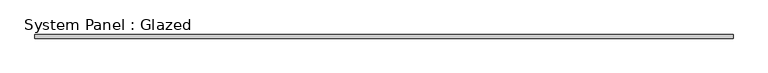
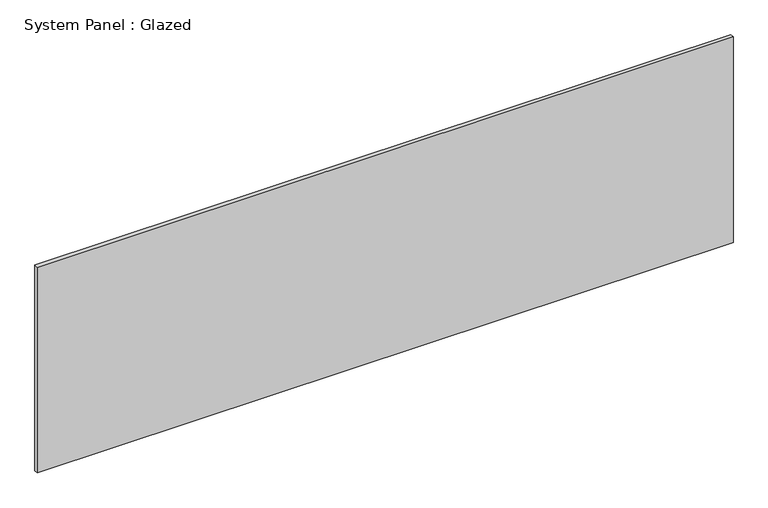
"""IFC4 building model written with IfcOpenShell, lengths in millimetres: plate geometry, System Panel : Glazed."""

from ifc_helpers import new_model, si_unit, origin, origin_with_axes, place, context, project, spatial, polyline, outline, extrude, source, transform, mapped, element, save


def system_panel_glazed_6303489a(model_context):
    return source(origin(), model_context, "Body", "SweptSolid", [
        extrude(outline(polyline([(2438.4, 19.05), (-2438.4, 19.05), (-2438.4, 44.45), (2438.4, 44.45), (2438.4, 19.05)])), origin_with_axes(), (0.0, 0.0, 1.0), 1524.0),
    ])


if __name__ == "__main__":
    model = new_model("IFC4")
    model_context = context("Model", 3, world=origin())
    ifc_project = project(units=[si_unit("LENGTHUNIT", "METRE", prefix="MILLI")], contexts=[model_context])
    site = spatial("IfcSite", under=ifc_project)
    building = spatial("IfcBuilding", under=site)
    placement = place(None, origin())
    system_panel_glazed_shape = system_panel_glazed_6303489a(model_context)
    element("IfcPlate", 1, ObjectType="System Panel : Glazed", at=placement, inside=building, context=model_context, shape_type="MappedRepresentation", body=[
        mapped(system_panel_glazed_shape, transform((0.0, 0.0, 0.0), x_axis=(1.0, 0.0, 0.0), y_axis=(0.0, 1.0, 0.0), z_axis=(0.0, 0.0, 1.0))),
    ])
    save(model, "model.ifc")

# Revit data of these elements
# Type "System Panel : Glazed"
#   Construction Type Id = "GSP4R"
#   Analytic Construction = "1/8 in Pilkington single glazing"
#   Visual Light Transmittance = 0.9
#   Solar Heat Gain Coefficient = 0.86
#   Heat Transfer Coefficient (U) = 1.18115 BTU/(h·ft²·°F)
# Element 1 (IfcPlate, "System Panel : Glazed")
#   Materials on its faces: "Glass"
# Materials
#   "Glass": class "Glass", colour RGB 0 128 192, transparency 0.75, Description = "Soda Lime Glass", Cost = 0
